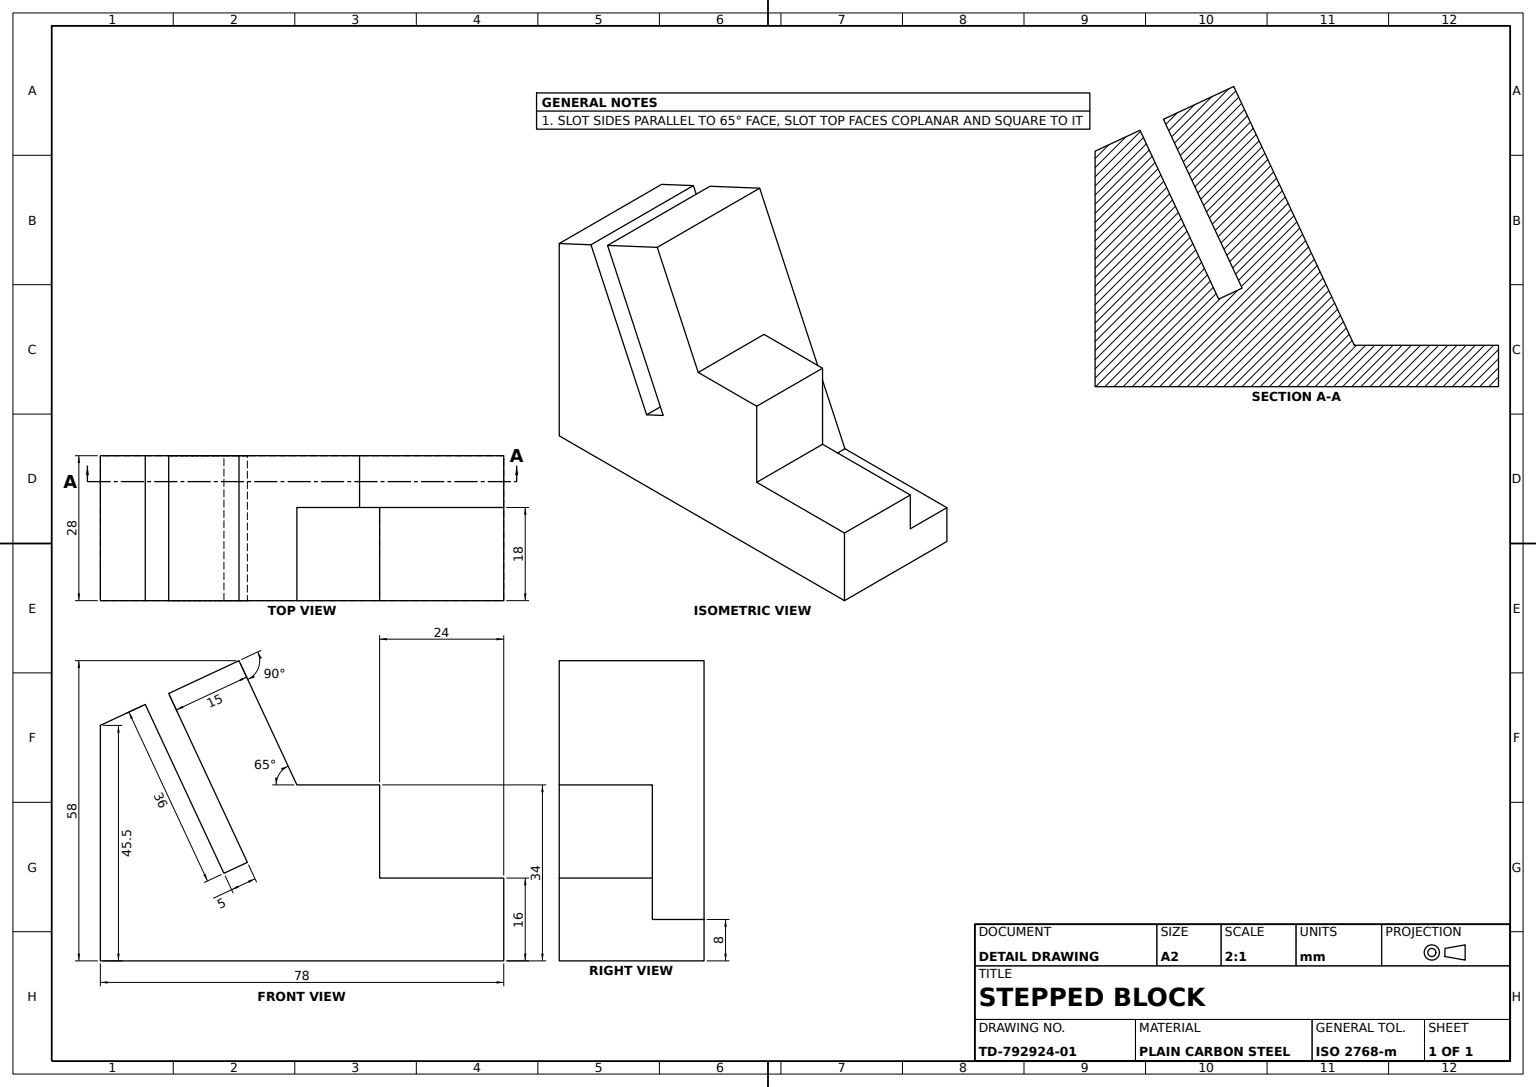
from build123d import *

# Parameters (mm, degrees)
BASE_PLATE_SKETCH_W      = 78
BASE_PLATE_SKETCH_H      = 28
BASE_PLATE_78X28X8_DEPTH = 8
STEP_BLOCK_DEPTH         = 18
V_NOTCH_UPRIGHT_REACH    = 60.83


with BuildPart() as part:
    # Base Plate Sketch → Base Plate 78x28x8 (new body)
    with BuildSketch(Plane(origin=(0, 0, 0), x_dir=(1, 0, 0), z_dir=(0, 1, 0))):
        Rectangle(BASE_PLATE_SKETCH_W, BASE_PLATE_SKETCH_H)
    extrude(amount=BASE_PLATE_78X28X8_DEPTH)

    # Step Block Sketch → Step Block (add)
    with BuildSketch(Plane(origin=(0, 0, -14), x_dir=(-1, 0, 0), z_dir=(0, 0, -1))):
        Polygon((39, 8), (39, 16), (15, 16), (15, 34), (-1, 34), (-1, 8), align=None)
    extrude(amount=-STEP_BLOCK_DEPTH)

    # V-Notch Upright: up to this face of the body (flat: up to its plane)
    v_notch_upright_end = Plane(part.part.faces().sort_by_distance((-6.571428571, 10.987012987, -14))[0])
    # V-Notch Upright Sketch → V-Notch Upright (add, up to the picked face)
    with BuildSketch(Plane.XY.offset(14), mode=Mode.PRIVATE) as v_notch_upright_sk1:
        Polygon((-11.123999112, 8), (12.191383796, 58), (25.786000601, 51.660726074), (10.571743179, 19.033645741), (15.103282114, 16.920554432), (30.317539536, 49.547634765), (39, 45.498936959), (39, 8), align=None)
    v_notch_upright_tool1 = split(extrude(v_notch_upright_sk1.sketch, amount=-V_NOTCH_UPRIGHT_REACH, mode=Mode.PRIVATE), bisect_by=v_notch_upright_end, keep=Keep.BOTH, mode=Mode.PRIVATE)
    add(v_notch_upright_tool1.solids().sort_by(Axis((1.175344, 32.700793, 14), (0, 0, -1)))[0])


solid = part.part
